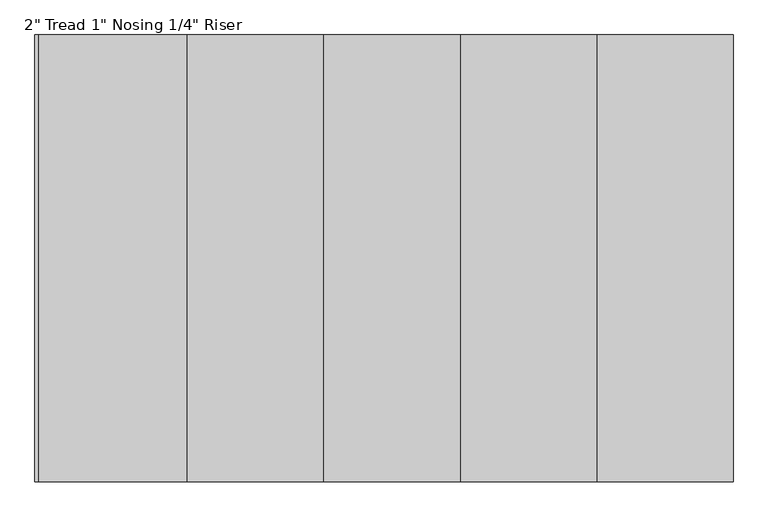
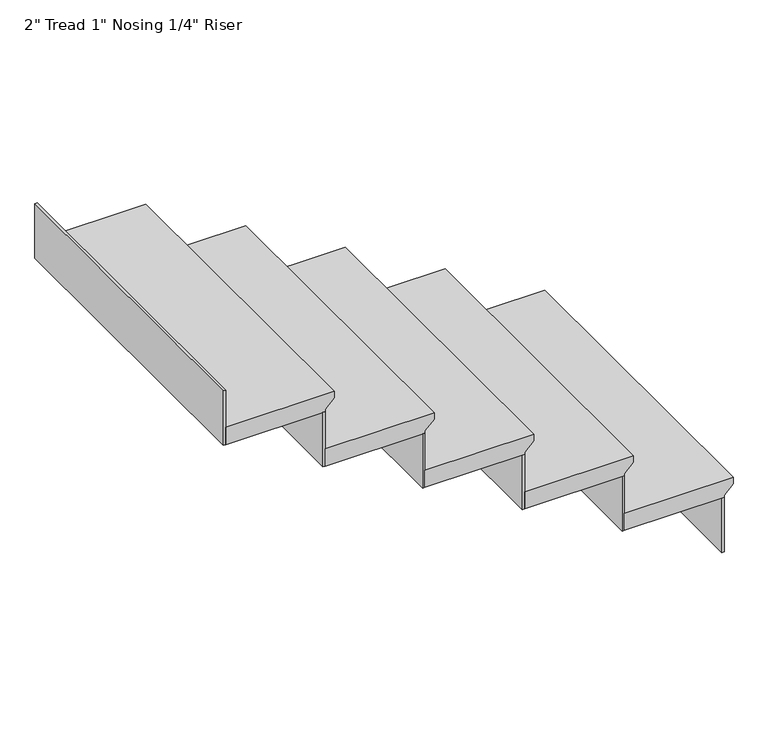
"""IFC4 building model written with IfcOpenShell, lengths in millimetres: stair flight geometry."""

from ifc_helpers import new_model, si_unit, frame, origin, place, context, project, spatial, polyline, outline, extrude, source, transform, mapped, element, save


def stair_flight_b9a180af(model_context):
    return source(origin(), model_context, "Body", "SweptSolid", [
        extrude(outline(polyline([(2241.1764706, 2644.5430349), (2241.1764706, 2339.7430349), (2190.3764706, 2339.7430349), (2190.3764706, 2619.1430349), (2196.7264706, 2619.1430349), (2222.1264706, 2644.5430349), (2241.1764706, 2644.5430349)])), frame((0.0, 2083.4555142, 0.0), z_axis=(0.0, 1.0, 0.0), x_axis=(0.0, 0.0, 1.0)), (0.0, 0.0, 1.0), 914.4),
        extrude(outline(polyline([(2612.7930349, 2997.8555142), (2619.1430349, 2997.8555142), (2619.1430349, 2083.4555142), (2612.7930349, 2083.4555142), (2612.7930349, 2997.8555142)])), frame((0.0, 0.0, 2029.0117647), z_axis=(0.0, 0.0, 1.0), x_axis=(1.0, 0.0, 0.0)), (0.0, 0.0, 1.0), 161.3647059),
        extrude(outline(polyline([(2333.3930349, 2997.8555142), (2339.7430349, 2997.8555142), (2339.7430349, 2083.4555142), (2333.3930349, 2083.4555142), (2333.3930349, 2997.8555142)])), frame((0.0, 0.0, 2190.3764706), z_axis=(0.0, 0.0, 1.0), x_axis=(1.0, 0.0, 0.0)), (0.0, 0.0, 1.0), 161.3647059),
        extrude(outline(polyline([(2402.5411765, 2365.1430349), (2402.5411765, 2060.3430349), (2351.7411765, 2060.3430349), (2351.7411765, 2339.7430349), (2358.0911765, 2339.7430349), (2383.4911765, 2365.1430349), (2402.5411765, 2365.1430349)])), frame((0.0, 2083.4555142, 0.0), z_axis=(0.0, 1.0, 0.0), x_axis=(0.0, 0.0, 1.0)), (0.0, 0.0, 1.0), 914.4),
        extrude(outline(polyline([(2053.9930349, 2997.8555142), (2060.3430349, 2997.8555142), (2060.3430349, 2083.4555142), (2053.9930349, 2083.4555142), (2053.9930349, 2997.8555142)])), frame((0.0, 0.0, 2351.7411765), z_axis=(0.0, 0.0, 1.0), x_axis=(1.0, 0.0, 0.0)), (0.0, 0.0, 1.0), 161.3647059),
        extrude(outline(polyline([(2563.9058824, 2085.7430349), (2563.9058824, 1780.9430349), (2513.1058824, 1780.9430349), (2513.1058824, 2060.3430349), (2519.4558824, 2060.3430349), (2544.8558824, 2085.7430349), (2563.9058824, 2085.7430349)])), frame((0.0, 2083.4555142, 0.0), z_axis=(0.0, 1.0, 0.0), x_axis=(0.0, 0.0, 1.0)), (0.0, 0.0, 1.0), 914.4),
        extrude(outline(polyline([(1774.5930349, 2997.8555142), (1780.9430349, 2997.8555142), (1780.9430349, 2083.4555142), (1774.5930349, 2083.4555142), (1774.5930349, 2997.8555142)])), frame((0.0, 0.0, 2513.1058824), z_axis=(0.0, 0.0, 1.0), x_axis=(1.0, 0.0, 0.0)), (0.0, 0.0, 1.0), 161.3647059),
        extrude(outline(polyline([(2725.2705882, 1806.3430349), (2725.2705882, 1501.5430349), (2674.4705882, 1501.5430349), (2674.4705882, 1780.9430349), (2680.8205882, 1780.9430349), (2706.2205882, 1806.3430349), (2725.2705882, 1806.3430349)])), frame((0.0, 2083.4555142, 0.0), z_axis=(0.0, 1.0, 0.0), x_axis=(0.0, 0.0, 1.0)), (0.0, 0.0, 1.0), 914.4),
        extrude(outline(polyline([(1495.1930349, 2997.8555142), (1501.5430349, 2997.8555142), (1501.5430349, 2083.4555142), (1495.1930349, 2083.4555142), (1495.1930349, 2997.8555142)])), frame((0.0, 0.0, 2674.4705882), z_axis=(0.0, 0.0, 1.0), x_axis=(1.0, 0.0, 0.0)), (0.0, 0.0, 1.0), 161.3647059),
        extrude(outline(polyline([(1215.7930349, 2997.8555142), (1222.1430349, 2997.8555142), (1222.1430349, 2083.4555142), (1215.7930349, 2083.4555142), (1215.7930349, 2997.8555142)])), frame((0.0, 0.0, 2835.8352941), z_axis=(0.0, 0.0, 1.0), x_axis=(1.0, 0.0, 0.0)), (0.0, 0.0, 1.0), 161.3647059),
        extrude(outline(polyline([(2886.6352941, 1526.9430349), (2886.6352941, 1222.1430349), (2835.8352941, 1222.1430349), (2835.8352941, 1501.5430349), (2842.1852941, 1501.5430349), (2867.5852941, 1526.9430349), (2886.6352941, 1526.9430349)])), frame((0.0, 2083.4555142, 0.0), z_axis=(0.0, 1.0, 0.0), x_axis=(0.0, 0.0, 1.0)), (0.0, 0.0, 1.0), 914.4),
    ])


if __name__ == "__main__":
    model = new_model("IFC4")
    model_context = context("Model", 3, world=origin())
    ifc_project = project(units=[si_unit("LENGTHUNIT", "METRE", prefix="MILLI")], contexts=[model_context])
    site = spatial("IfcSite", under=ifc_project)
    building = spatial("IfcBuilding", under=site)
    placement = place(None, origin())
    stair_flight_shape = stair_flight_b9a180af(model_context)
    element("IfcStairFlight", 1, ObjectType="2\" Tread 1\" Nosing 1/4\" Riser", at=placement, inside=building, context=model_context, shape_type="MappedRepresentation", body=[
        mapped(stair_flight_shape, transform((0.0, 0.0, 0.0), x_axis=(1.0, 0.0, 0.0), y_axis=(0.0, 1.0, 0.0), z_axis=(0.0, 0.0, 1.0))),
    ])
    save(model, "model.ifc")
